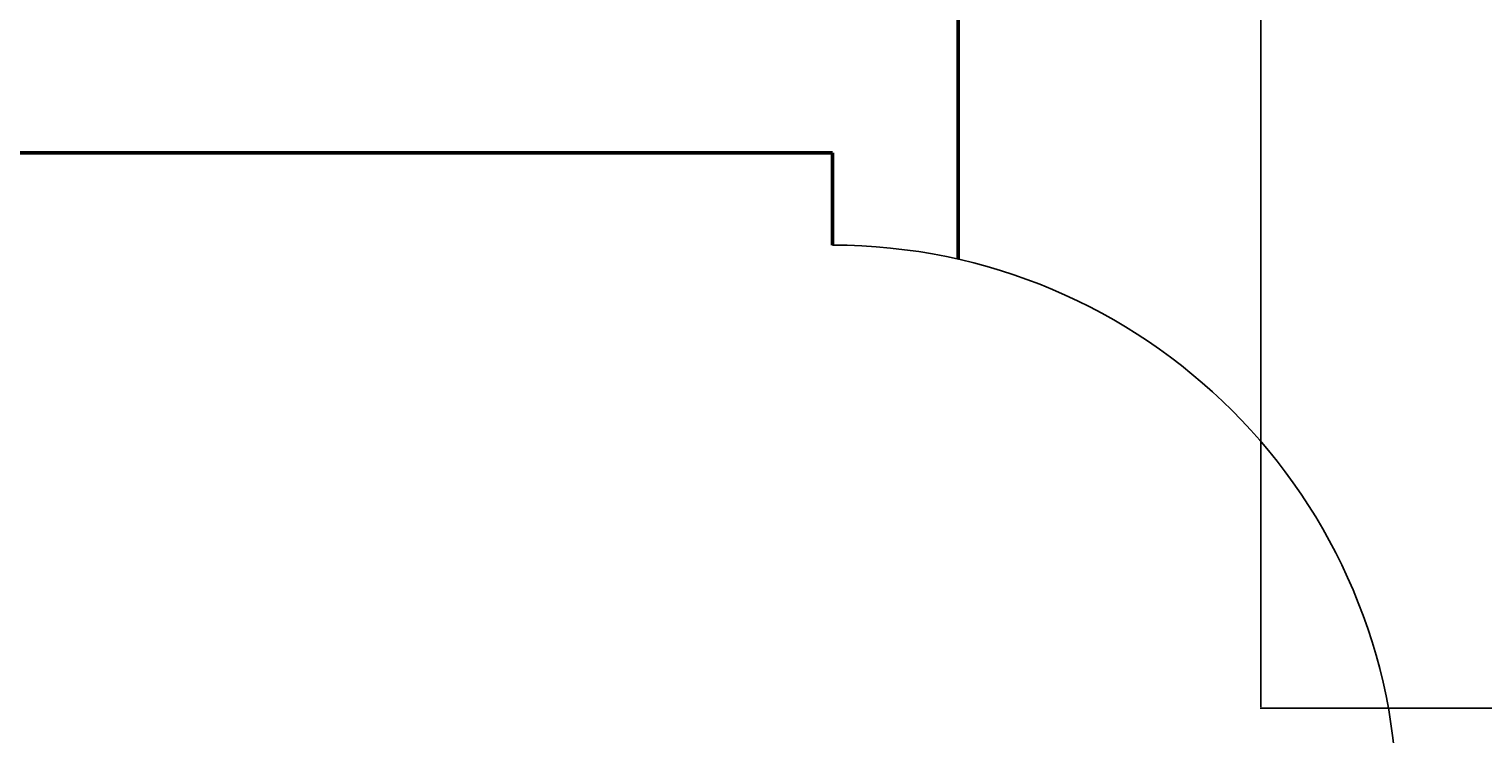
# Model space of a CAD drawing. Units: millimetres. Extents: x -857 to 54106, y -13666 to 13947.
# Tile 22 of 41: x 28540 to 30856, y 8428 to 9552. Entities that reach past the tile are written whole.
import ezdxf

# ---------------------------------------------------------------- set-up
doc = ezdxf.new("R2010")
doc.units = ezdxf.units.MM
for name, color, linetype, lineweight in [('A-ANNO-DIMS', 2, 'Continuous', 18), ('A-DOOR', 1, 'Continuous', 25), ('A-WALL', 7, 'Continuous', 50)]:
    doc.layers.add(name, color=color, linetype=linetype, lineweight=lineweight)
doc.styles.get("Standard").update_dxf_attribs({"font": 'arial.ttf'})
doc.dimstyles.new('ISO-25', dxfattribs={"dimtxt": 2.5, "dimasz": 2.5, "dimexe": 1.25, "dimexo": 0.625, "dimtad": 1, "dimtxsty": 'Standard', "dimcen": 2.5, "dimadec": 0, "dimazin": 0, "dimtfac": 1, "dimtmove": 0, "dimatfit": 3, "dimfxl": 1, "dimarcsym": 0})

# ---------------------------------------------------------------- blocks, each defined once
blk = doc.blocks.new('DOOR-900')
blk.add_line((11417.3, 9811.5), (12317.3, 9811.5))
blk.add_arc((11417.3, 9811.5), 900, 0, 90)
blk = doc.blocks.new('*D48')
at = {"layer": 'A-ANNO-DIMS', "color": 0, "lineweight": -2, "transparency": 16777216}
for p, q in [((30908.6, 11089.5), (30501.4, 11089.5)), ((30502.6, 11087), (30502.6, 8471.5)), ((30908.6, 8469), (30501.4, 8469))]:
    blk.add_line(p, q, dxfattribs=at)
at = {"layer": 'A-ANNO-DIMS', "color": 0, "transparency": 16777216}
for points in [[(30502.2, 11087), (30503, 11087), (30502.6, 11089.5)], [(30502.2, 8471.5), (30503, 8471.5), (30502.6, 8469)]]:
    blk.add_solid(points, dxfattribs=at)
at = {"layer": 'Defpoints', "color": 0, "transparency": 16777216}
for p in [(30909.3, 11089.5), (30502.6, 8469), (30909.3, 8469)]:
    blk.add_point(p, dxfattribs=at)
at = {"layer": 'A-ANNO-DIMS', "color": 0, "transparency": 16777216, "insert": (30500.7, 9779.2), "char_height": 2.5, "attachment_point": 5, "rotation": 90}
blk.add_mtext('2620 TYP.', dxfattribs=at)

msp = doc.modelspace()

# ---------------------------------------------------------------- linework, layer by layer
at = {"layer": 'A-WALL'}
for p, q in [((30020.079, 11404.231), (30020.079, 9184.795)), ((27216.59, 9354.231), (29820.079, 9354.231)), ((29820.079, 9207.298), (29820.079, 9354.231))]:
    msp.add_line(p, q, dxfattribs=at)

# ---------------------------------------------------------------- block references
at = {"layer": 'A-DOOR'}
msp.add_blockref('DOOR-900', (18402.799, -1504.183), dxfattribs=at)

# ---------------------------------------------------------------- dimensions: what is measured, and where the dimension line sits
at = {"layer": 'A-ANNO-DIMS'}
dim = msp.add_linear_dim(base=(30502.63, 8468.999), p1=(30909.254, 11089.463), p2=(30909.254, 8468.999), angle=270, text='<> TYP.', dimstyle='ISO-25', override={"dimdec": 0, "dimrnd": 0, "dimzin": 0, "dimlunit": 2}, dxfattribs=at)
dim.commit()
dim.dimension.update_dxf_attribs({"geometry": '*D48', "text_midpoint": (30500.728, 9779.231)})

doc.saveas('drawing.dxf')
